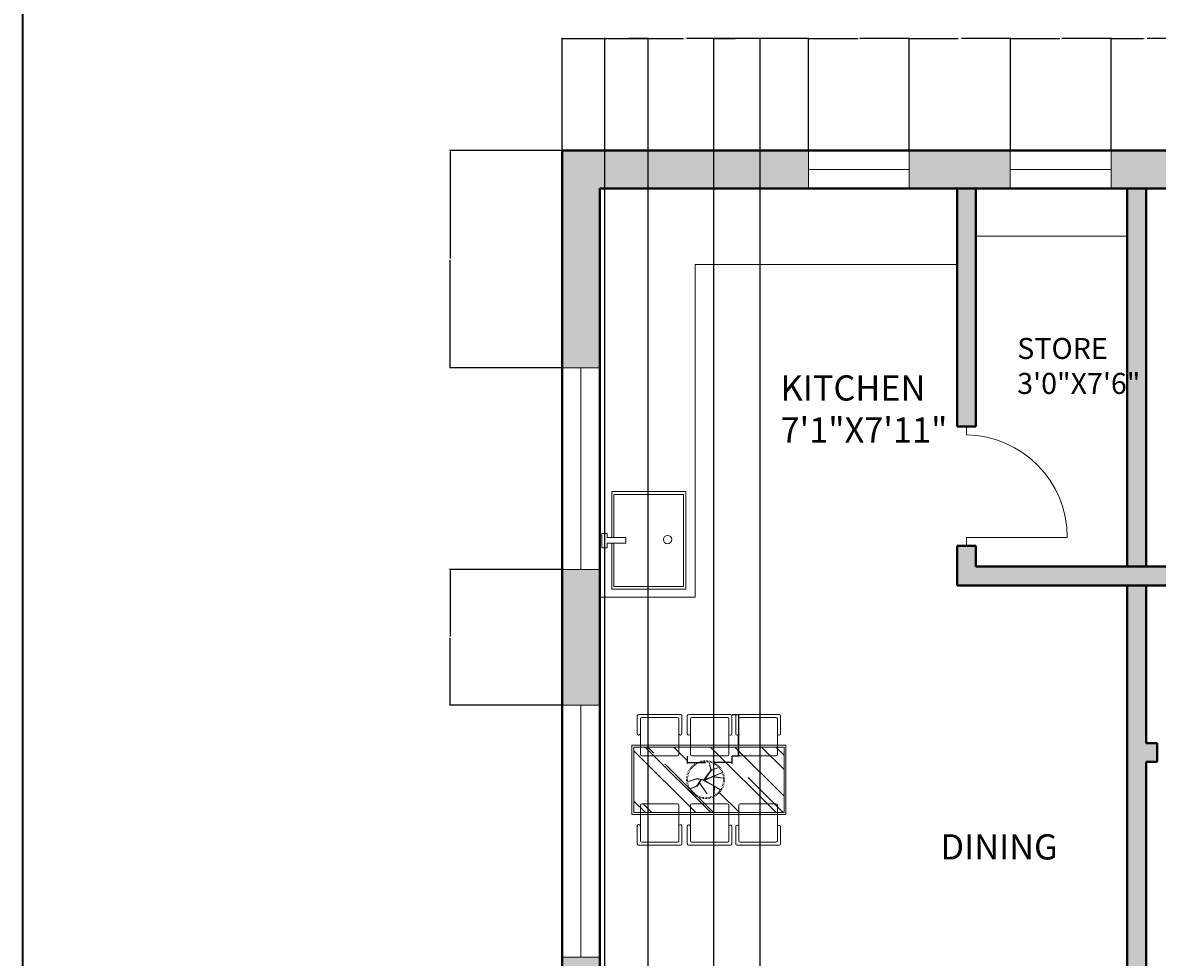
# Model space of a CAD drawing. Units: inches. Extents: x 1441 to 2460, y 1648 to 2683.
# Tile 12 of 35: x 1441 to 1711, y 2107 to 2329. Entities that reach past the tile are written whole.
import ezdxf

# ---------------------------------------------------------------- set-up
doc = ezdxf.new("R2010")
doc.units = ezdxf.units.IN
for name, color, linetype, lineweight in [('A-ANNO-DIMS', 2, 'Continuous', 18), ('A-ANNO-TTLB', 7, 'Continuous', 35), ('A-AREA-IDEN', 7, 'Continuous', 20), ('A-DOOR', 3, 'Continuous', 20), ('A-FLOR-CASE', 9, 'Continuous', 20), ('A-FLOR-FIXT', 9, 'Continuous', 18), ('A-FURN', 8, 'Continuous', 15), ('A-FURN-PATT', 252, 'Continuous', 9), ('A-GLAZ', 4, 'Continuous', 18), ('A-WALL', 7, 'Continuous', 40)]:
    doc.layers.add(name, color=color, linetype=linetype, lineweight=lineweight)
doc.layers.add('A-WALL-PATT', color=251, linetype='Continuous', lineweight=13, true_color=0x636466)
doc.styles.get("Standard").update_dxf_attribs({"font": 'arial.ttf'})
doc.dimstyles.get("Standard").update_dxf_attribs({"dimtxt": 0.18, "dimasz": 0.18, "dimexe": 0.18, "dimexo": 0.0625, "dimgap": 0.09, "dimtad": 0, "dimtih": 1, "dimtoh": 1, "dimdec": 4, "dimzin": 0, "dimdsep": 46, "dimtxsty": 'Standard', "dimcen": 0.09, "dimadec": 0, "dimazin": 0, "dimtfac": 1, "dimtdec": 4, "dimtofl": 0, "dimtmove": 0, "dimatfit": 3, "dimfxl": 1, "dimtolj": 1, "dimtzin": 0, "dimarcsym": 0})

# ---------------------------------------------------------------- blocks, each defined once
blk = doc.blocks.new('DOOR-STORE-24')
for p, q in [((0, 28.42), (0, 26.42)), ((0, 0), (0, 2)), ((0, 2), (24, 2))]:
    blk.add_line(p, q)
blk.add_arc((-0.43, 2), 24.43, 0, 88.9938)
blk = doc.blocks.new('WIN-48-SASH')
for p, q in [((9, 48), (4.5, 48)), ((4.5, 48), (4.5, 0)), ((4.5, 0), (0, 0))]:
    blk.add_line(p, q)
blk = doc.blocks.new('WIN-60-SASH')
for p, q in [((9, 60), (4.5, 60)), ((4.5, 60), (4.5, 0)), ((4.5, 0), (0, 0))]:
    blk.add_line(p, q)
blk = doc.blocks.new('SINK-KITCHEN')
for points in [[(2.36, 12.29), (2.36, 23.19), (19.96, 23.19), (19.96, 0), (2.36, 0), (2.36, 10.91)], [(2.84, 12.29), (2.84, 22.51), (19.43, 22.51), (19.43, 0.62), (2.84, 0.62), (2.84, 10.91)], [(1.21, 10.91), (1.21, 9.78), (0, 9.78), (0, 13.22), (1.21, 13.22), (1.21, 12.29)], [(1.21, 12.29), (5.65, 12.29), (5.65, 10.91), (1.21, 10.91)]]:
    blk.add_lwpolyline(points)
blk.add_circle((15.62, 11.79), 0.997)
blk = doc.blocks.new('DINING-CHAIR')
for p, q in [((0, 5.27), (0, 9.54)), ((0.33, 9.87), (10.3, 9.87)), ((0.73, 8.81), (0.73, 0.33)), ((1.06, 9.14), (9.57, 9.14)), ((9.9, 8.81), (9.9, 0.33)), ((10.63, 9.54), (10.63, 5.27)), ((0.33, 4.94), (0.4, 4.94)), ((10.23, 4.94), (10.3, 4.94)), ((1.06, 0), (9.57, 0))]:
    blk.add_line(p, q)
for centre, start, end in [((0.33, 9.54), 90, 180), ((1.06, 8.81), 90, 180), ((9.57, 8.81), 0, 90), ((10.3, 9.54), 0, 90), ((0.33, 5.27), 180, 270), ((0.4, 5.27), 270, 0), ((10.23, 5.27), 180, 270), ((10.3, 5.27), 270, 0), ((1.06, 0.33), 180, 270), ((9.57, 0.33), 270, 0)]:
    blk.add_arc(centre, 0.33, start, end)
blk = doc.blocks.new('*D38')
at = {"layer": 'A-ANNO-DIMS', "color": 0, "lineweight": -2, "transparency": 16777216}
for p, q in [((1598.69, 2154.57), (1598.69, 2152.86)), ((1598.87, 2153.04), (1603.05, 2153.04)), ((1609.14, 2153.04), (1604.96, 2153.04)), ((1609.32, 2154.57), (1609.32, 2152.86))]:
    blk.add_line(p, q, dxfattribs=at)
at = {"layer": 'A-ANNO-DIMS', "color": 0, "transparency": 16777216}
for points in [[(1598.87, 2153.07), (1598.87, 2153.01), (1598.69, 2153.04)], [(1609.14, 2153.07), (1609.14, 2153.01), (1609.32, 2153.04)]]:
    blk.add_solid(points, dxfattribs=at)
at = {"layer": 'Defpoints', "color": 0, "transparency": 16777216}
for p in [(1598.69, 2154.63), (1609.32, 2154.63), (1609.32, 2153.04)]:
    blk.add_point(p, dxfattribs=at)
at = {"layer": 'A-ANNO-DIMS', "color": 0, "transparency": 16777216, "insert": (1604.01, 2153.04), "char_height": 0.18, "attachment_point": 5}
blk.add_mtext('\\A1;CHAIR 11 TYP.', dxfattribs=at)
blk = doc.blocks.new('*D39')
at = {"layer": 'A-ANNO-DIMS', "color": 0, "lineweight": -2, "transparency": 16777216}
for p, q in [((1609.39, 2164.5), (1611.1, 2164.5)), ((1610.92, 2164.32), (1610.92, 2159.75)), ((1610.92, 2154.81), (1610.92, 2159.38)), ((1609.39, 2154.63), (1611.1, 2154.63))]:
    blk.add_line(p, q, dxfattribs=at)
at = {"layer": 'A-ANNO-DIMS', "color": 0, "transparency": 16777216}
for points in [[(1610.89, 2164.32), (1610.95, 2164.32), (1610.92, 2164.5)], [(1610.89, 2154.81), (1610.95, 2154.81), (1610.92, 2154.63)]]:
    blk.add_solid(points, dxfattribs=at)
at = {"layer": 'Defpoints', "color": 0, "transparency": 16777216}
for p in [(1609.32, 2164.5), (1610.92, 2164.5), (1609.32, 2154.63)]:
    blk.add_point(p, dxfattribs=at)
at = {"layer": 'A-ANNO-DIMS', "color": 0, "transparency": 16777216, "insert": (1610.92, 2159.57), "char_height": 0.18, "attachment_point": 5}
blk.add_mtext('\\A1;10 TYP.', dxfattribs=at)
blk = doc.blocks.new('*D68')
at = {"layer": 'A-ANNO-DIMS', "color": 0, "lineweight": -2, "transparency": 16777216}
for p, q in [((1568.89, 2298.76), (1568.89, 2325.53)), ((1569.07, 2325.35), (1597.8, 2325.35)), ((1627.33, 2325.35), (1598.59, 2325.35)), ((1627.51, 2298.76), (1627.51, 2325.53))]:
    blk.add_line(p, q, dxfattribs=at)
at = {"layer": 'A-ANNO-DIMS', "color": 0, "transparency": 16777216}
for points in [[(1569.07, 2325.38), (1569.07, 2325.32), (1568.89, 2325.35)], [(1627.33, 2325.38), (1627.33, 2325.32), (1627.51, 2325.35)]]:
    blk.add_solid(points, dxfattribs=at)
at = {"layer": 'Defpoints', "color": 0, "transparency": 16777216}
for p in [(1627.51, 2325.35), (1568.89, 2298.7), (1627.51, 2298.7)]:
    blk.add_point(p, dxfattribs=at)
at = {"layer": 'A-ANNO-DIMS', "color": 0, "transparency": 16777216, "insert": (1598.2, 2325.35), "char_height": 0.18, "attachment_point": 5}
blk.add_mtext('\\A1;58.62', dxfattribs=at)
blk = doc.blocks.new('*D69')
at = {"layer": 'A-ANNO-DIMS', "color": 0, "lineweight": -2, "transparency": 16777216}
for p, q in [((1627.51, 2298.76), (1627.51, 2325.53)), ((1627.69, 2325.35), (1639.29, 2325.35)), ((1651.33, 2325.35), (1639.73, 2325.35)), ((1651.51, 2298.76), (1651.51, 2325.53))]:
    blk.add_line(p, q, dxfattribs=at)
at = {"layer": 'A-ANNO-DIMS', "color": 0, "transparency": 16777216}
for points in [[(1627.69, 2325.38), (1627.69, 2325.32), (1627.51, 2325.35)], [(1651.33, 2325.38), (1651.33, 2325.32), (1651.51, 2325.35)]]:
    blk.add_solid(points, dxfattribs=at)
at = {"layer": 'Defpoints', "color": 0, "transparency": 16777216}
for p in [(1651.51, 2325.35), (1627.51, 2298.7), (1651.51, 2298.7)]:
    blk.add_point(p, dxfattribs=at)
at = {"layer": 'A-ANNO-DIMS', "color": 0, "transparency": 16777216, "insert": (1639.51, 2325.35), "char_height": 0.18, "attachment_point": 5}
blk.add_mtext('\\A1;24', dxfattribs=at)
blk = doc.blocks.new('*D70')
at = {"layer": 'A-ANNO-DIMS', "color": 0, "lineweight": -2, "transparency": 16777216}
for p, q in [((1651.51, 2298.76), (1651.51, 2325.53)), ((1651.69, 2325.35), (1663.15, 2325.35)), ((1675.4, 2325.35), (1663.94, 2325.35)), ((1675.58, 2298.76), (1675.58, 2325.53))]:
    blk.add_line(p, q, dxfattribs=at)
at = {"layer": 'A-ANNO-DIMS', "color": 0, "transparency": 16777216}
for points in [[(1651.69, 2325.38), (1651.69, 2325.32), (1651.51, 2325.35)], [(1675.4, 2325.38), (1675.4, 2325.32), (1675.58, 2325.35)]]:
    blk.add_solid(points, dxfattribs=at)
at = {"layer": 'Defpoints', "color": 0, "transparency": 16777216}
for p in [(1675.58, 2325.35), (1651.51, 2298.7), (1675.58, 2298.7)]:
    blk.add_point(p, dxfattribs=at)
at = {"layer": 'A-ANNO-DIMS', "color": 0, "transparency": 16777216, "insert": (1663.54, 2325.35), "char_height": 0.18, "attachment_point": 5}
blk.add_mtext('\\A1;24.07', dxfattribs=at)
blk = doc.blocks.new('*D71')
at = {"layer": 'A-ANNO-DIMS', "color": 0, "lineweight": -2, "transparency": 16777216}
for p, q in [((1675.58, 2298.76), (1675.58, 2325.53)), ((1675.76, 2325.35), (1687.36, 2325.35)), ((1699.4, 2325.35), (1687.8, 2325.35)), ((1699.58, 2298.76), (1699.58, 2325.53))]:
    blk.add_line(p, q, dxfattribs=at)
at = {"layer": 'A-ANNO-DIMS', "color": 0, "transparency": 16777216}
for points in [[(1675.76, 2325.38), (1675.76, 2325.32), (1675.58, 2325.35)], [(1699.4, 2325.38), (1699.4, 2325.32), (1699.58, 2325.35)]]:
    blk.add_solid(points, dxfattribs=at)
at = {"layer": 'Defpoints', "color": 0, "transparency": 16777216}
for p in [(1699.58, 2325.35), (1675.58, 2298.7), (1699.58, 2298.7)]:
    blk.add_point(p, dxfattribs=at)
at = {"layer": 'A-ANNO-DIMS', "color": 0, "transparency": 16777216, "insert": (1687.58, 2325.35), "char_height": 0.18, "attachment_point": 5}
blk.add_mtext('\\A1;24', dxfattribs=at)
blk = doc.blocks.new('*D72')
at = {"layer": 'A-ANNO-DIMS', "color": 0, "lineweight": -2, "transparency": 16777216}
for p, q in [((1699.58, 2298.76), (1699.58, 2325.53)), ((1699.76, 2325.35), (1707.27, 2325.35)), ((1715.69, 2325.35), (1708.18, 2325.35)), ((1715.87, 2298.76), (1715.87, 2325.53))]:
    blk.add_line(p, q, dxfattribs=at)
at = {"layer": 'A-ANNO-DIMS', "color": 0, "transparency": 16777216}
for points in [[(1699.76, 2325.38), (1699.76, 2325.32), (1699.58, 2325.35)], [(1715.69, 2325.38), (1715.69, 2325.32), (1715.87, 2325.35)]]:
    blk.add_solid(points, dxfattribs=at)
at = {"layer": 'Defpoints', "color": 0, "transparency": 16777216}
for p in [(1715.87, 2325.35), (1699.58, 2298.7), (1715.87, 2298.7)]:
    blk.add_point(p, dxfattribs=at)
at = {"layer": 'A-ANNO-DIMS', "color": 0, "transparency": 16777216, "insert": (1707.72, 2325.35), "char_height": 0.18, "attachment_point": 5}
blk.add_mtext('\\A1;16.294', dxfattribs=at)
blk = doc.blocks.new('*D78')
at = {"layer": 'A-ANNO-DIMS', "color": 0, "lineweight": -2, "transparency": 16777216}
for p, q in [((1568.82, 2198.96), (1542.06, 2198.96)), ((1542.24, 2198.78), (1542.24, 2183.01)), ((1542.24, 2166.87), (1542.24, 2182.64)), ((1568.82, 2166.69), (1542.06, 2166.69))]:
    blk.add_line(p, q, dxfattribs=at)
at = {"layer": 'A-ANNO-DIMS', "color": 0, "transparency": 16777216}
for points in [[(1542.21, 2198.78), (1542.27, 2198.78), (1542.24, 2198.96)], [(1542.21, 2166.87), (1542.27, 2166.87), (1542.24, 2166.69)]]:
    blk.add_solid(points, dxfattribs=at)
at = {"layer": 'Defpoints', "color": 0, "transparency": 16777216}
for p in [(1542.24, 2198.96), (1568.89, 2198.96), (1568.89, 2166.69)]:
    blk.add_point(p, dxfattribs=at)
at = {"layer": 'A-ANNO-DIMS', "color": 0, "transparency": 16777216, "insert": (1542.24, 2182.83), "char_height": 0.18, "attachment_point": 5}
blk.add_mtext('\\A1;32.27', dxfattribs=at)
blk = doc.blocks.new('*D79')
at = {"layer": 'A-ANNO-DIMS', "color": 0, "lineweight": -2, "transparency": 16777216}
for p, q in [((1568.82, 2298.7), (1542.06, 2298.7)), ((1542.24, 2298.52), (1542.24, 2273.01)), ((1542.24, 2247.14), (1542.24, 2272.65)), ((1568.82, 2246.96), (1542.06, 2246.96))]:
    blk.add_line(p, q, dxfattribs=at)
at = {"layer": 'A-ANNO-DIMS', "color": 0, "transparency": 16777216}
for points in [[(1542.21, 2298.52), (1542.27, 2298.52), (1542.24, 2298.7)], [(1542.21, 2247.14), (1542.27, 2247.14), (1542.24, 2246.96)]]:
    blk.add_solid(points, dxfattribs=at)
at = {"layer": 'Defpoints', "color": 0, "transparency": 16777216}
for p in [(1542.24, 2298.7), (1568.89, 2298.7), (1568.89, 2246.96)]:
    blk.add_point(p, dxfattribs=at)
at = {"layer": 'A-ANNO-DIMS', "color": 0, "transparency": 16777216, "insert": (1542.24, 2272.83), "char_height": 0.18, "attachment_point": 5}
blk.add_mtext('\\A1;51.73', dxfattribs=at)
blk = doc.blocks.new('*D124')
at = {"layer": 'A-ANNO-DIMS', "color": 0, "lineweight": -2, "transparency": 16777216}
for p, q in [((1604.98, 2008.16), (1604.98, 2325.53)), ((1605.16, 2325.35), (1610.06, 2325.35)), ((1615.87, 2325.35), (1610.97, 2325.35)), ((1616.05, 2008.16), (1616.05, 2325.53))]:
    blk.add_line(p, q, dxfattribs=at)
at = {"layer": 'A-ANNO-DIMS', "color": 0, "transparency": 16777216}
for points in [[(1605.16, 2325.38), (1605.16, 2325.32), (1604.98, 2325.35)], [(1615.87, 2325.38), (1615.87, 2325.32), (1616.05, 2325.35)]]:
    blk.add_solid(points, dxfattribs=at)
at = {"layer": 'Defpoints', "color": 0, "transparency": 16777216}
for p in [(1616.05, 2325.35), (1604.98, 2008.09), (1616.05, 2008.09)]:
    blk.add_point(p, dxfattribs=at)
at = {"layer": 'A-ANNO-DIMS', "color": 0, "transparency": 16777216, "insert": (1610.51, 2325.35), "char_height": 0.18, "attachment_point": 5}
blk.add_mtext('\\A1;11.075', dxfattribs=at)
blk = doc.blocks.new('*D126')
at = {"layer": 'A-ANNO-DIMS', "color": 0, "lineweight": -2, "transparency": 16777216}
for p, q in [((1579.1, 2036.67), (1579.1, 2325.53)), ((1579.28, 2325.35), (1583.77, 2325.35)), ((1589.17, 2325.35), (1584.68, 2325.35)), ((1589.35, 2036.78), (1589.35, 2325.53))]:
    blk.add_line(p, q, dxfattribs=at)
at = {"layer": 'A-ANNO-DIMS', "color": 0, "transparency": 16777216}
for points in [[(1579.28, 2325.38), (1579.28, 2325.32), (1579.1, 2325.35)], [(1589.17, 2325.38), (1589.17, 2325.32), (1589.35, 2325.35)]]:
    blk.add_solid(points, dxfattribs=at)
at = {"layer": 'Defpoints', "color": 0, "transparency": 16777216}
for p in [(1589.35, 2325.35), (1579.1, 2036.6), (1589.35, 2036.72)]:
    blk.add_point(p, dxfattribs=at)
at = {"layer": 'A-ANNO-DIMS', "color": 0, "transparency": 16777216, "insert": (1584.23, 2325.35), "char_height": 0.18, "attachment_point": 5}
blk.add_mtext('\\A1;10.253', dxfattribs=at)

msp = doc.modelspace()

# ---------------------------------------------------------------- hatches: boundary and pattern name
at = {"layer": 'A-FURN-PATT'}
h = msp.add_hatch(dxfattribs=at)
h.set_pattern_fill('AR-RROOF', color=256, scale=11.004311, angle=-45, style=0)
h.set_pattern_definition([(315, (1947.642, 3073.833), (24.89991, -9.33747), [165.0647, -22.0086, 55.0216, -11.0043]), (315, (1961.882, 3067.374), (2.5678, 18.13025), [33.0129, -3.6314, 66.0259, -8.2532]), (315, (1958.1466, 3076.556), (45.67578, -35.24894), [88.0345, -15.40604, 44.01724, -11.0043])])
h.paths.add_polyline_path([(1585.9462, 2141.1291), (1621.7102, 2141.1291), (1621.7102, 2156.7185), (1585.9462, 2156.7185)])
at = {"layer": 'A-WALL-PATT'}
h = msp.add_hatch(color=256, dxfattribs=at)
h.dxf.hatch_style = 1
h.paths.add_polyline_path([(1627.5085, 2298.6952), (1568.8859, 2298.6952), (1568.8859, 2246.9605), (1577.8859, 2246.9605), (1577.8859, 2289.6952), (1627.5085, 2289.6952), (1627.5085, 2294.1952)])
h.paths.add_polyline_path([(1675.5777, 2298.6952), (1651.5085, 2298.6952), (1651.5085, 2289.6952), (1675.5777, 2289.6952), (1675.5777, 2294.1952)])
h.paths.add_polyline_path([(1667.3859, 2289.6952), (1662.8859, 2289.6952), (1662.8859, 2233.0622), (1667.3859, 2233.0622)])
h.paths.add_polyline_path([(1715.8721, 2294.3362), (1715.8721, 2295.2788), (1715.8721, 2298.6952), (1699.5777, 2298.6952), (1699.5777, 2289.6952), (1715.8721, 2289.6952)])
h.paths.add_polyline_path([(1707.8859, 2289.6952), (1703.3859, 2289.6952), (1703.3859, 2199.6952), (1707.8859, 2199.6952)])
h.paths.add_polyline_path([(1760.3859, 2204.637), (1755.8859, 2204.637), (1755.8859, 2199.6952), (1667.3859, 2199.6952), (1667.3859, 2204.637), (1662.8859, 2204.637), (1662.8859, 2195.1952), (1760.3859, 2195.1952)])
h.paths.add_polyline_path([(1760.3859, 2289.6952), (1755.8859, 2289.6952), (1755.8859, 2233.0622), (1760.3859, 2233.0622)])
h.paths.add_polyline_path([(1889.3859, 2298.6952), (1739.8721, 2298.6952), (1739.8721, 2289.6952), (1880.3859, 2289.6952), (1880.3859, 2250.8051), (1889.3859, 2250.8051)])
h.paths.add_polyline_path([(1889.3859, 2202.8051), (1880.3859, 2202.8051), (1880.3859, 2157.6952), (1747.948, 2157.6952), (1747.948, 2153.1952), (1755.8859, 2153.1952), (1755.8859, 2058.005), (1760.3859, 2058.005), (1760.3859, 2153.1952), (1880.3859, 2153.1952), (1880.3859, 2124.108), (1889.3859, 2124.108)])
h.paths.add_polyline_path([(1889.3859, 1984.8305), (1880.3859, 1984.8305), (1880.3859, 1834.1952), (1889.3859, 1834.1952)])
h.paths.add_polyline_path([(1889.3859, 2076.108), (1880.3859, 2076.108), (1880.3859, 2008.8305), (1889.3859, 2008.8305)])
h.paths.add_polyline_path([(1880.3859, 2027.1952), (1800.8859, 2027.1952), (1800.8859, 2000.9452), (1805.3859, 2000.9452), (1805.3859, 2022.6952), (1880.3859, 2022.6952)])
h.paths.add_polyline_path([(1800.8859, 2027.1952), (1760.3859, 2027.1952), (1760.3859, 2030.7912), (1755.8859, 2030.7912), (1755.8859, 2022.6952), (1800.8859, 2022.6952)])
h.paths.add_polyline_path([(1880.3859, 1974.6952), (1805.3859, 1974.6952), (1805.3859, 1978.7973), (1800.8859, 1978.7973), (1800.8859, 1974.6952), (1794.8823, 1974.6952), (1794.8823, 1970.1952), (1800.8859, 1970.1952), (1805.3859, 1970.1952), (1880.3859, 1970.1952)])
h.paths.add_polyline_path([(1760.3859, 1974.6952), (1755.8859, 1974.6952), (1755.8859, 1925.6952), (1751.8616, 1925.6952), (1751.8616, 1921.1952), (1760.3859, 1921.1952)])
h.paths.add_polyline_path([(1760.3859, 1921.1952), (1755.8859, 1921.1952), (1755.8859, 1843.1952), (1760.3859, 1843.1952)])
h.paths.add_polyline_path([(1799.1136, 1838.6952), (1799.1136, 1843.1952), (1760.3859, 1843.1952), (1751.8944, 1843.1952), (1751.8944, 1834.1952), (1758.1615, 1834.1952), (1799.1136, 1834.1952)])
h.paths.add_polyline_path([(1880.3859, 1843.1952), (1859.1136, 1843.1952), (1859.1136, 1834.1952), (1880.3859, 1834.1952)])
h.paths.add_polyline_path([(1577.8859, 1857.7914), (1568.8859, 1857.7914), (1568.8859, 1834.1952), (1695.0034, 1834.1952), (1695.0034, 1838.6952), (1695.0034, 1843.1952), (1577.8859, 1843.1952)])
h.paths.add_polyline_path([(1577.8859, 1959.2399), (1573.3859, 1959.2399), (1568.8859, 1959.2399), (1568.8859, 1905.7914), (1577.8859, 1905.7914), (1577.8859, 1921.1952), (1703.3859, 1921.1952), (1707.8859, 1921.1952), (1715.1501, 1921.1952), (1715.1501, 1925.6952), (1707.8859, 1925.6952), (1703.3859, 1925.6952), (1577.8859, 1925.6952)])
h.paths.add_polyline_path([(1577.8859, 2106.6907), (1568.8859, 2106.6907), (1568.8859, 2019.2399), (1577.8859, 2019.2399)])
h.paths.add_polyline_path([(1707.8859, 2051.6952), (1703.3859, 2051.6952), (1703.3859, 2048.6952), (1703.3859, 1925.6952), (1707.8859, 1925.6952)])
h.paths.add_polyline_path([(1703.3859, 2051.6952), (1676.3859, 2051.6952), (1676.3859, 2048.6952), (1703.3859, 2048.6952)])
h.paths.add_polyline_path([(1703.3859, 2102.6952), (1676.3859, 2102.6952), (1676.3859, 2099.6952), (1685.3859, 2099.6952), (1703.3859, 2099.6952)])
h.paths.add_polyline_path([(1707.8859, 2153.1952), (1710.5611, 2153.1952), (1710.5611, 2157.6952), (1707.8859, 2157.6952), (1707.8859, 2195.1952), (1703.3859, 2195.1952), (1703.3859, 2099.6952), (1707.8859, 2099.6952)])
h.paths.add_polyline_path([(1577.8859, 2198.9605), (1568.8859, 2198.9605), (1568.8859, 2166.6907), (1577.8859, 2166.6907)])

# ---------------------------------------------------------------- linework, layer by layer
at = {"layer": 'A-ANNO-TTLB'}
msp.add_lwpolyline([(1440.5107, 2682.6413), (2460.193, 2682.6413), (2460.193, 1648.08), (1440.5107, 1648.08)], close=True, dxfattribs=at)
at = {"layer": 'A-FLOR-CASE'}
for p, q in [((1667.3859, 2278.307), (1703.3859, 2278.307)), ((1600.573, 2192.432), (1600.573, 2271.5733)), ((1600.573, 2271.5733), (1662.8859, 2271.5733)), ((1577.8859, 2192.432), (1584.8606, 2192.432)), ((1584.8606, 2192.432), (1600.573, 2192.432))]:
    msp.add_line(p, q, dxfattribs=at)
at = {"layer": 'A-FURN'}
for p, q in [((1586.7886, 2159.8967), (1586.7886, 2164.1702)), ((1587.1188, 2164.5004), (1597.096, 2164.5004)), ((1587.5222, 2163.4366), (1587.5222, 2154.9628)), ((1587.8524, 2163.7667), (1596.3624, 2163.7667)), ((1596.6925, 2163.4366), (1596.6925, 2154.9628)), ((1597.4261, 2164.1702), (1597.4261, 2159.8967)), ((1587.1188, 2159.5665), (1587.1921, 2159.5665)), ((1597.0226, 2159.5665), (1597.096, 2159.5665)), ((1622.1687, 2157.177), (1585.4877, 2157.177)), ((1585.4877, 2157.177), (1585.4877, 2140.6706)), ((1621.7102, 2156.7185), (1585.9462, 2156.7185)), ((1585.9462, 2156.7185), (1585.9462, 2141.1291)), ((1621.7102, 2141.1291), (1621.7102, 2156.7185)), ((1622.1687, 2140.6706), (1622.1687, 2157.177)), ((1587.8524, 2154.6327), (1596.3624, 2154.6327)), ((1600.1339, 2152.0368), (1599.8817, 2152.3032)), ((1600.3832, 2152.2549), (1600.1526, 2152.5403)), ((1600.6488, 2152.4528), (1600.4413, 2152.7554)), ((1600.9291, 2152.6293), (1600.746, 2152.9471)), ((1601.2224, 2152.7832), (1601.0648, 2153.1144)), ((1601.5268, 2152.9136), (1601.3958, 2153.2562)), ((1601.8406, 2153.0197), (1601.7368, 2153.3715)), ((1602.1617, 2153.1009), (1602.0858, 2153.4598)), ((1602.4882, 2153.1566), (1602.4407, 2153.5204)), ((1602.8181, 2153.1866), (1602.7993, 2153.5529)), ((1603.1493, 2153.1906), (1603.1593, 2153.5572)), ((1603.4798, 2153.1685), (1603.5185, 2153.5333)), ((1603.8075, 2153.1207), (1603.8747, 2153.4812)), ((1603.9953, 2152.8754), (1604.2901, 2151.171)), ((1604.3556, 2151.2365), (1603.9953, 2152.8754)), ((1604.1305, 2153.0472), (1604.2258, 2153.4014)), ((1604.4467, 2152.9486), (1604.5695, 2153.2943)), ((1604.7542, 2152.8256), (1604.9038, 2153.1605)), ((1605.0511, 2152.6787), (1605.2265, 2153.0009)), ((1605.3356, 2152.5091), (1605.5357, 2152.8165)), ((1605.6058, 2152.3176), (1605.8295, 2152.6084)), ((1605.8603, 2152.1056), (1606.106, 2152.3779)), ((1598.8874, 2149.7471), (1598.5268, 2149.8143)), ((1598.9609, 2150.07), (1598.6067, 2150.1653)), ((1599.0594, 2150.3862), (1598.7138, 2150.5091)), ((1599.1825, 2150.6937), (1598.8476, 2150.8433)), ((1599.3293, 2150.9907), (1599.0072, 2151.166)), ((1599.499, 2151.2751), (1599.1916, 2151.4752)), ((1599.6904, 2151.5454), (1599.3997, 2151.769)), ((1599.9025, 2151.7998), (1599.6302, 2152.0456)), ((1604.2901, 2151.171), (1602.5541, 2148.8767)), ((1607.0414, 2150.6466), (1602.5541, 2148.8767)), ((1602.7506, 2148.7783), (1604.6851, 2149.6206)), ((1602.7834, 2148.9094), (1604.3883, 2151.171)), ((1605.9933, 2151.761), (1604.3556, 2151.2365)), ((1604.3883, 2151.171), (1605.9933, 2151.761)), ((1607.2052, 2149.3355), (1604.6851, 2149.6206)), ((1604.856, 2149.6951), (1607.0414, 2150.6466)), ((1604.856, 2149.6951), (1607.2052, 2149.3355)), ((1606.0973, 2151.8742), (1606.3636, 2152.1264)), ((1606.3154, 2151.6249), (1606.6007, 2151.8554)), ((1606.5133, 2151.3593), (1606.8158, 2151.5667)), ((1606.6897, 2151.079), (1607.0076, 2151.262)), ((1606.8436, 2150.7857), (1607.1749, 2150.9432)), ((1606.974, 2150.4812), (1607.3166, 2150.6123)), ((1607.0802, 2150.1675), (1607.432, 2150.2713)), ((1607.1613, 2149.8464), (1607.5202, 2149.9222)), ((1598.8175, 2149.0888), (1598.4508, 2149.0988)), ((1598.8215, 2148.7576), (1598.4552, 2148.7388)), ((1598.8395, 2149.4193), (1598.4748, 2149.4581)), ((1598.8514, 2148.4278), (1598.4877, 2148.3803)), ((1598.9072, 2148.1013), (1598.5483, 2148.0254)), ((1598.9883, 2147.7801), (1598.6365, 2147.6763)), ((1601.0146, 2149.27), (1598.6891, 2148.4506)), ((1598.6891, 2148.4506), (1601.0146, 2149.1717)), ((1599.0945, 2147.4664), (1598.7519, 2147.3353)), ((1599.2249, 2147.1619), (1598.8936, 2147.0044)), ((1600.9819, 2147.5001), (1599.4097, 2146.779)), ((1599.4097, 2146.779), (1601.0801, 2147.4345)), ((1601.9645, 2149.0405), (1600.9819, 2147.5001)), ((1602.5541, 2148.9094), (1601.0146, 2149.27)), ((1601.0146, 2149.1717), (1602.7506, 2148.7456)), ((1601.0801, 2147.4345), (1601.9973, 2148.9422)), ((1603.4384, 2145.6318), (1601.5059, 2148.2211)), ((1601.6042, 2148.2211), (1603.4384, 2145.6318)), ((1605.0762, 2147.3887), (1602.5868, 2148.7456)), ((1602.7834, 2148.7783), (1606.6156, 2146.5496)), ((1605.0762, 2145.5991), (1605.0762, 2147.3887)), ((1605.1532, 2147.3467), (1605.0762, 2145.5991)), ((1606.6156, 2146.5496), (1605.1532, 2147.3467)), ((1606.7392, 2146.957), (1607.0614, 2146.7816)), ((1606.886, 2147.2539), (1607.2209, 2147.1043)), ((1607.0091, 2147.5614), (1607.3547, 2147.4386)), ((1607.1076, 2147.8776), (1607.4619, 2147.7823)), ((1607.1811, 2148.2006), (1607.5417, 2148.1333)), ((1607.2171, 2149.5199), (1607.5808, 2149.5673)), ((1607.229, 2148.5283), (1607.5937, 2148.4896)), ((1607.247, 2149.19), (1607.6134, 2149.2088)), ((1607.251, 2148.8588), (1607.6177, 2148.8488)), ((1599.3788, 2146.8686), (1599.0609, 2146.6856)), ((1599.5552, 2146.5883), (1599.2527, 2146.3809)), ((1599.7531, 2146.3227), (1599.4678, 2146.0922)), ((1599.9712, 2146.0734), (1599.7049, 2145.8212)), ((1600.2082, 2145.8421), (1599.9625, 2145.5697)), ((1600.4627, 2145.63), (1600.239, 2145.3392)), ((1600.7329, 2145.4385), (1600.5328, 2145.1311)), ((1601.0174, 2145.2689), (1600.842, 2144.9467)), ((1601.3143, 2145.1221), (1601.1648, 2144.7871)), ((1601.6218, 2144.999), (1601.499, 2144.6533)), ((1601.938, 2144.9004), (1601.8427, 2144.5462)), ((1602.261, 2144.827), (1602.1938, 2144.4664)), ((1602.5888, 2144.7791), (1602.55, 2144.4143)), ((1602.9192, 2144.7571), (1602.9092, 2144.3904)), ((1603.2504, 2144.761), (1603.2692, 2144.3947)), ((1603.5803, 2144.791), (1603.6278, 2144.4273)), ((1603.9068, 2144.8467), (1603.9827, 2144.4878)), ((1604.2279, 2144.9279), (1604.3317, 2144.5761)), ((1604.5417, 2145.034), (1604.6728, 2144.6914)), ((1604.8461, 2145.1644), (1605.0037, 2144.8332)), ((1605.1394, 2145.3183), (1605.3225, 2145.0005)), ((1605.4198, 2145.4948), (1605.6272, 2145.1923)), ((1605.6854, 2145.6927), (1605.9159, 2145.4074)), ((1605.9346, 2145.9108), (1606.1868, 2145.6444)), ((1606.166, 2146.1478), (1606.4383, 2145.902)), ((1606.3781, 2146.4022), (1606.6688, 2146.1786)), ((1606.5695, 2146.6725), (1606.8769, 2146.4724)), ((1587.5222, 2142.8848), (1587.5222, 2134.411)), ((1587.8524, 2143.2149), (1596.3624, 2143.2149)), ((1596.6925, 2134.411), (1596.6925, 2142.8848)), ((1599.4204, 2142.8848), (1599.4204, 2134.411)), ((1599.7505, 2143.2149), (1608.2605, 2143.2149)), ((1608.5907, 2134.411), (1608.5907, 2142.8848)), ((1610.9639, 2134.411), (1610.9639, 2142.8848)), ((1619.804, 2143.2149), (1611.294, 2143.2149)), ((1620.1341, 2142.8848), (1620.1341, 2134.411)), ((1585.4877, 2140.6706), (1622.1687, 2140.6706)), ((1585.9462, 2141.1291), (1621.7102, 2141.1291)), ((1586.7886, 2137.951), (1586.7886, 2133.6774)), ((1587.1209, 2138.2789), (1587.1943, 2138.2784)), ((1597.0246, 2138.2132), (1597.098, 2138.2128)), ((1597.4261, 2133.6774), (1597.4261, 2137.951)), ((1598.6868, 2137.951), (1598.6868, 2133.6774)), ((1599.0188, 2138.2), (1599.0922, 2138.1995)), ((1608.9225, 2138.1344), (1608.9958, 2138.1339)), ((1609.3243, 2133.6774), (1609.3243, 2137.951)), ((1610.2303, 2133.6774), (1610.2303, 2137.951)), ((1610.6354, 2138.123), (1610.5621, 2138.1235)), ((1620.5391, 2138.0574), (1620.4657, 2138.0579)), ((1620.8678, 2137.951), (1620.8678, 2133.6774)), ((1587.8524, 2134.0809), (1596.3624, 2134.0809)), ((1599.7505, 2134.0809), (1608.2605, 2134.0809)), ((1619.804, 2134.0809), (1611.294, 2134.0809)), ((1587.1188, 2133.3473), (1597.096, 2133.3473)), ((1599.0169, 2133.3473), (1608.9941, 2133.3473)), ((1620.5376, 2133.3473), (1610.5604, 2133.3473))]:
    msp.add_line(p, q, dxfattribs=at)
for centre, start, end in [((1587.1188, 2164.1702), 90, 180), ((1587.8524, 2163.4366), 90, 180), ((1596.3624, 2163.4366), 0, 90), ((1597.096, 2164.1702), 0, 90), ((1587.1188, 2159.8967), 180, 0.103974), ((1597.0226, 2159.8967), 180, 0.103974), ((1587.8524, 2154.9628), 180, 270), ((1596.3624, 2154.9628), 270, 0), ((1587.8524, 2142.8848), 90, 180), ((1596.3624, 2142.8848), 0, 90), ((1599.7505, 2142.8848), 90, 180), ((1608.2605, 2142.8848), 0, 90), ((1611.294, 2142.8848), 90, 180), ((1619.804, 2142.8848), 0, 90), ((1587.1188, 2137.9488), 89.620247, 179.620246), ((1587.1921, 2137.9483), 359.620246, 89.620247), ((1597.0224, 2137.8831), 89.620247, 179.620246), ((1597.0958, 2137.8826), 359.620246, 89.620247), ((1599.0166, 2137.8699), 89.620247, 179.620246), ((1599.09, 2137.8694), 359.620246, 89.620247), ((1608.9203, 2137.8043), 89.620247, 179.620246), ((1608.9937, 2137.8038), 359.620246, 89.620247), ((1610.5599, 2137.7934), 89.620247, 179.620246), ((1610.6332, 2137.7929), 359.620246, 89.620247), ((1620.4635, 2137.7278), 89.620247, 179.620246), ((1620.5369, 2137.7273), 359.620246, 89.620247), ((1587.1188, 2133.6774), 180, 270), ((1587.8524, 2134.411), 180, 270), ((1596.3624, 2134.411), 270, 0), ((1597.096, 2133.6774), 270, 0), ((1599.0169, 2133.6774), 180, 270), ((1599.7505, 2134.411), 180, 270), ((1608.2605, 2134.411), 270, 0), ((1608.9941, 2133.6774), 270, 0), ((1610.5604, 2133.6774), 180, 270), ((1611.294, 2134.411), 180, 270), ((1619.804, 2134.411), 270, 0), ((1620.5376, 2133.6774), 270, 0)]:
    msp.add_arc(centre, 0.3301, start, end, dxfattribs=at)
at = {"layer": 'A-GLAZ'}
for p, q in [((1627.5085, 2298.6952), (1627.5085, 2289.6952)), ((1651.5085, 2294.1952), (1651.5085, 2298.6952)), ((1651.5085, 2298.6952), (1651.5085, 2289.6952)), ((1675.5777, 2298.6952), (1675.5777, 2289.6952)), ((1699.5777, 2294.1952), (1699.5777, 2298.6952)), ((1699.5777, 2298.6952), (1699.5777, 2289.6952)), ((1627.5085, 2289.6952), (1627.5085, 2294.1952)), ((1627.5085, 2294.1952), (1651.5085, 2294.1952)), ((1675.5777, 2289.6952), (1675.5777, 2294.1952)), ((1675.5777, 2294.1952), (1699.5777, 2294.1952)), ((1568.8859, 2246.9605), (1577.8859, 2246.9605)), ((1568.8859, 2198.9605), (1577.8859, 2198.9605)), ((1568.8859, 2166.6907), (1577.8859, 2166.6907)), ((1568.8859, 2106.6907), (1577.8859, 2106.6907))]:
    msp.add_line(p, q, dxfattribs=at)
at = {"layer": 'A-WALL'}
for p, q in [((1568.8859, 2298.6952), (1568.8859, 1834.1952)), ((1568.8859, 2298.6952), (1889.3859, 2298.6952)), ((1577.8859, 2289.6952), (1880.3859, 2289.6952)), ((1577.8859, 2289.6952), (1577.8859, 2157.6952)), ((1577.8859, 2289.6952), (1577.8859, 1925.6952)), ((1662.8859, 2289.6952), (1662.8859, 2233.0622)), ((1667.3859, 2289.6952), (1667.3859, 2233.0622)), ((1703.3859, 2289.6952), (1703.3859, 2199.6952)), ((1707.8859, 2289.6952), (1707.8859, 2199.6952)), ((1662.8859, 2233.0622), (1667.3859, 2233.0622)), ((1667.3859, 2204.637), (1662.8859, 2204.637)), ((1662.8859, 2204.637), (1662.8859, 2195.1952)), ((1667.3859, 2204.637), (1667.3859, 2199.6952)), ((1667.3859, 2199.6952), (1755.8859, 2199.6952)), ((1662.8859, 2195.1952), (1760.3859, 2195.1952)), ((1703.3859, 2195.1952), (1703.3859, 2099.6952)), ((1707.8859, 2195.1952), (1707.8859, 2157.6952)), ((1707.8859, 2157.6952), (1710.5611, 2157.6952)), ((1710.5611, 2157.6952), (1710.5611, 2153.1952)), ((1707.8859, 2153.1952), (1710.5611, 2153.1952)), ((1707.8859, 2153.1952), (1707.8859, 2099.6952))]:
    msp.add_line(p, q, dxfattribs=at)

# ---------------------------------------------------------------- block references
at = {"layer": 'A-DOOR'}
msp.add_blockref('DOOR-STORE-24', (1665.14, 2204.64), dxfattribs=at)
at = {"layer": 'A-FLOR-FIXT'}
msp.add_blockref('SINK-KITCHEN', (1578.38, 2194.34), dxfattribs=at)
at = {"layer": 'A-FURN'}
for p in [(1598.69, 2154.63), (1610.2335, 2154.63)]:
    msp.add_blockref('DINING-CHAIR', p, dxfattribs=at)
at = {"layer": 'A-GLAZ'}
for name, p in [('WIN-48-SASH', (1568.89, 2198.96)), ('WIN-60-SASH', (1568.89, 2106.69))]:
    msp.add_blockref(name, p, dxfattribs=at)

# ---------------------------------------------------------------- texts
at = {"layer": 'A-AREA-IDEN', "attachment_point": 1}
for s, insert, char_height in [('STORE\\P3\'0"X7\'6"', (1677.2195, 2254.1105), 5), ('KITCHEN\\P7\'1"X7\'11"', (1620.8816, 2245.2042), 6), ('DINING', (1658.9488, 2135.9799), 6)]:
    msp.add_mtext_dynamic_manual_height_columns(s, width=85.554017, gutter_width=12.5, heights=[0], dxfattribs=dict(at, insert=insert, char_height=char_height))

# ---------------------------------------------------------------- dimensions: what is measured, and where the dimension line sits
at = {"layer": 'A-ANNO-DIMS'}
for base, p1, p2, override, picture, middle in [((1627.5085, 2325.3452), (1568.8859, 2298.6952), (1627.5085, 2298.6952), {"dimdec": 2, "dimlfac": 1, "dimrnd": 0, "dimzin": 0, "dimdsep": 46, "dimlunit": 2}, '*D68', (1598.1972, 2325.3452)), ((1589.3522, 2325.3452), (1579.099, 2036.6042), (1589.3522, 2036.7181), {"dimdec": 3, "dimlfac": 1, "dimrnd": 0, "dimzin": 0, "dimdsep": 46, "dimlunit": 2}, '*D126', (1584.2256, 2325.3452)), ((1616.0509, 2325.3452), (1604.9763, 2008.0936), (1616.0509, 2008.0936), {"dimdec": 3, "dimlfac": 1, "dimrnd": 0, "dimzin": 0, "dimdsep": 46, "dimlunit": 2}, '*D124', (1610.5136, 2325.3452)), ((1651.5085, 2325.3452), (1627.5085, 2298.6952), (1651.5085, 2298.6952), {"dimdec": 0, "dimlfac": 1, "dimrnd": 0, "dimzin": 0, "dimdsep": 46, "dimlunit": 2}, '*D69', (1639.5085, 2325.3452)), ((1675.5777, 2325.3452), (1651.5085, 2298.6952), (1675.5777, 2298.6952), {"dimdec": 2, "dimlfac": 1, "dimrnd": 0, "dimzin": 0, "dimdsep": 46, "dimlunit": 2}, '*D70', (1663.5431, 2325.3452)), ((1699.5777, 2325.3452), (1675.5777, 2298.6952), (1699.5777, 2298.6952), {"dimdec": 0, "dimlfac": 1, "dimrnd": 0, "dimzin": 0, "dimdsep": 46, "dimlunit": 2}, '*D71', (1687.5777, 2325.3452)), ((1715.8721, 2325.3452), (1699.5777, 2298.6952), (1715.8721, 2298.6952), {"dimdec": 3, "dimlfac": 1, "dimrnd": 0, "dimzin": 0, "dimdsep": 46, "dimlunit": 2}, '*D72', (1707.7249, 2325.3452))]:
    dim = msp.add_linear_dim(base=base, p1=p1, p2=p2, dimstyle='Standard', override=override, dxfattribs=at)
    dim.commit()
    dim.dimension.update_dxf_attribs({"geometry": picture, "text_midpoint": middle})
for base, p1, p2, picture, middle in [((1542.2359, 2298.6952), (1568.8859, 2246.9605), (1568.8859, 2298.6952), '*D79', (1542.2359, 2272.8279)), ((1542.2359, 2198.9605), (1568.8859, 2166.6907), (1568.8859, 2198.9605), '*D78', (1542.2359, 2182.8256))]:
    dim = msp.add_linear_dim(base=base, p1=p1, p2=p2, angle=90, dimstyle='Standard', override={"dimdec": 2, "dimlfac": 1, "dimrnd": 0, "dimzin": 0, "dimdsep": 46, "dimlunit": 2}, dxfattribs=at)
    dim.commit()
    dim.dimension.update_dxf_attribs({"geometry": picture, "text_midpoint": middle})
dim = msp.add_linear_dim(base=(1610.9199, 2164.5004), p1=(1609.3243, 2154.6327), p2=(1609.3243, 2164.5004), angle=90, text='<> TYP.', dimstyle='Standard', override={"dimdec": 0, "dimlfac": 1, "dimrnd": 0, "dimzin": 0, "dimdsep": 46, "dimlunit": 2}, dxfattribs=at)
dim.commit()
dim.dimension.update_dxf_attribs({"geometry": '*D39', "text_midpoint": (1610.9199, 2159.5665)})
dim = msp.add_linear_dim(base=(1609.3243, 2153.0371), p1=(1598.6868, 2154.6327), p2=(1609.3243, 2154.6327), text='CHAIR <> TYP.', dimstyle='Standard', override={"dimdec": 0, "dimlfac": 1, "dimrnd": 0, "dimzin": 0, "dimdsep": 46, "dimlunit": 2}, dxfattribs=at)
dim.commit()
dim.dimension.update_dxf_attribs({"geometry": '*D38', "text_midpoint": (1604.0055, 2153.0371)})

doc.saveas('drawing.dxf')
